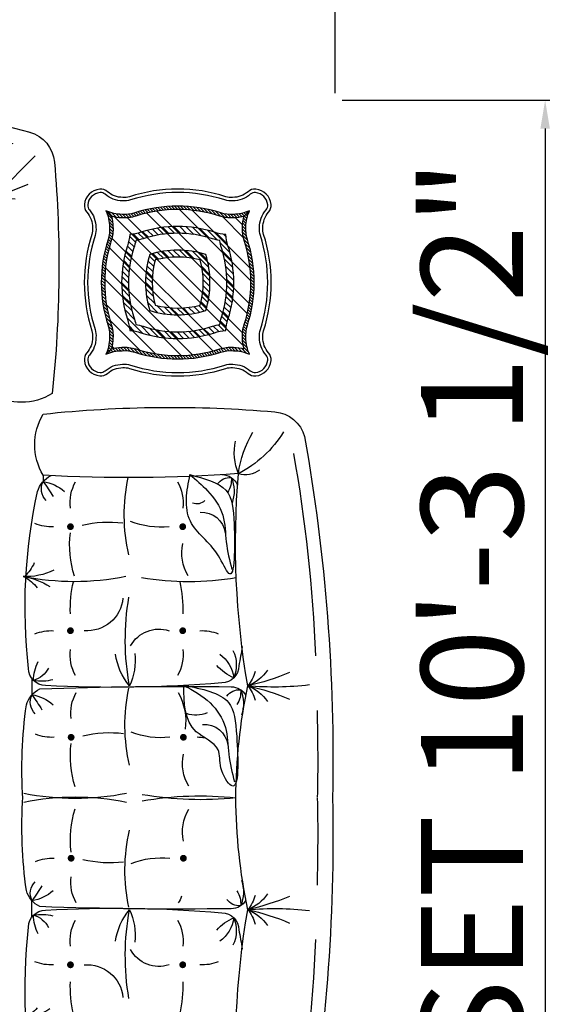
# Model space of a CAD drawing. Units: inches. Extents: x 3592 to 4861, y 1650 to 2243.
# Tile 10 of 30: x 4219 to 4265, y 1916 to 2003. Entities that reach past the tile are written whole.
import ezdxf

# ---------------------------------------------------------------- set-up
doc = ezdxf.new("R2010")
doc.units = ezdxf.units.IN
doc.layers.add('A-ANNO-DIMS', color=2, linetype='Continuous', lineweight=13)
doc.layers.add('A-FURN', color=9, linetype='Continuous', lineweight=13)
doc.layers.add('RA-AP-01$0$FURN', color=3, linetype='Continuous')
doc.layers.add('RA-AP-01$0$WOOD', color=64, linetype='Continuous')
doc.styles.get("Standard").update_dxf_attribs({"font": 'arial.ttf'})
doc.dimstyles.new('ISO-25', dxfattribs={"dimtxt": 9, "dimasz": 2.5, "dimexe": 1.25, "dimexo": 0.625, "dimtad": 1, "dimlunit": 3, "dimtxsty": 'Standard', "dimcen": 2.5, "dimadec": 0, "dimazin": 0, "dimtfac": 1, "dimtmove": 0, "dimatfit": 3, "dimfxl": 1, "dimarcsym": 0})
pattern_1 = [(225, (10.907943, -14.206733), (0.008838835, -0.008838835), [])]
pattern_2 = [(225, (10.9079426, -14.206733), (0.0044194174, -0.0044194174), [])]

# ---------------------------------------------------------------- blocks, each defined once
blk = doc.blocks.new('A$C6E322C05')
at = {"layer": 'RA-AP-01$0$FURN'}
for p, q in [((6.3919, -6.482), (6.5167, -6.3573)), ((6.3919, -6.482), (6.4334, -6.3775)), ((6.3919, -6.482), (6.3904, -6.4155)), ((5.8172, -6.4867), (5.8172, -6.5051)), ((6.3919, -6.482), (6.4393, -6.4682)), ((5.7672, -7.0775), (5.7672, -7.1067)), ((5.7672, -7.1359), (5.7672, -7.1067)), ((5.8172, -7.7267), (5.8172, -7.7084))]:
    blk.add_line(p, q, dxfattribs=at)
at = {"layer": 'RA-AP-01$0$FURN', "const_width": 0.01}
for points in [[(5.9025, -6.6381, 1), (5.8925, -6.6381, 1)], [(6.2228, -6.6381, -1), (6.2328, -6.6381, -1)], [(5.9025, -6.9444, -1), (5.8925, -6.9444, -1)], [(6.2228, -6.9444, 1), (6.2328, -6.9444, 1)], [(5.9025, -7.269, 1), (5.8925, -7.269, 1)], [(6.2228, -7.269, -1), (6.2328, -7.269, -1)], [(5.9025, -7.5753, -1), (5.8925, -7.5753, -1)], [(6.2228, -7.5753, 1), (6.2328, -7.5753, 1)]]:
    blk.add_lwpolyline(points, format="xyb", close=True, dxfattribs=at)
at = {"layer": 'RA-AP-01$0$FURN'}
for centre, radius, start, end in [((6.1922, -9.8397), 3.5528, 85.0473, 96.0589), ((5.9622, -6.3967), 0.1707, 148.1726, 211.8274), ((6.4903, -6.3998), 0.1, 15.4995, 85.0473), ((4.3367, -6.997), 2.3349, 357.3064, 15.4995), ((4.8466, -6.9097), 1.7752, 356.478, 15.9335), ((5.8573, -6.535), 0.05, 90, 180), ((6.0683, -2.0198), 4.4739, 266.7829, 274.1477), ((6.343, -6.535), 0.05, 22.5827, 90), ((8.747, -6.6855), 2.3639, 175.063, 189.8434), ((5.86, -6.527), 0.0479, 152.8071, 225.4025), ((5.7982, -6.6254), 0.1219, 48.0376, 81.0462), ((4.9043, -7.1366), 1.1102, 31.9329, 34.6665), ((6.0178, -6.5669), 0.1214, 150.1419, 187.6917), ((6.134, -6.5955), 0.1215, 123.1053, 153.7006), ((6.5659, -6.6031), 0.5101, 167.6182, 193.3122), ((6.1475, -6.4635), 0.0853, 200.7831, 253.0462), ((6.1075, -6.5669), 0.1214, 352.3083, 29.8581), ((6.3679, -6.5411), 0.0479, 86.5753, 142.6834), ((6.3027, -6.4996), 0.0683, 326.673, 5.2184), ((6.2748, -6.5339), 0.1042, 340.4828, 22.8693), ((7.0946, -6.9193), 1.3435, 163.3777, 185.4807), ((6.2698, -6.5402), 0.031, 245.776, 317.3789), ((6.2843, -6.6645), 0.0689, 6.4195, 94.4616), ((5.8396, -6.5171), 0.1213, 247.3376, 273.7315), ((6.0116, -6.9762), 0.3517, 83.4125, 103.1675), ((6.1623, -6.3952), 0.2442, 248.9017, 275.9924), ((6.1975, -6.6925), 0.3024, 173.0945, 197.5881), ((6.3545, -6.7151), 0.1295, 167.9901, 211.3796), ((5.6503, -6.6735), 0.1579, 315.4052, 333.0845), ((5.7659, -6.5936), 0.1916, 267.5853, 295.5831), ((5.9088, -6.0346), 0.7655, 258.6273, 281.4174), ((5.7331, -6.9697), 0.1864, 56.2926, 82.3818), ((5.6794, -6.9201), 0.1579, 40.3865, 58.0658), ((6.2458, -6.8794), 0.3487, 166.8392, 182.4658), ((6.2459, -5.9772), 0.8233, 260.2449, 279.7551), ((5.8795, -6.8794), 0.3487, 357.5342, 13.1608), ((5.9595, -6.8591), 0.093, 293.6025, 6.6107), ((6.8074, -6.9716), 0.7485, 170.3094, 190.3986), ((5.8396, -7.0655), 0.1213, 86.2685, 112.6624), ((5.9673, -7.035), 0.0954, 28.8034, 108.2253), ((6.158, -7.035), 0.0954, 71.7747, 151.1966), ((6.2857, -7.0655), 0.1213, 67.3376, 93.7315), ((6.0178, -7.0157), 0.1214, 172.3083, 209.8581), ((6.1075, -7.0157), 0.1214, 330.1419, 7.6917), ((6.28, -7.0949), 0.0991, 6.9226, 55.1088), ((6.2863, -7.0456), 0.0993, 337.9047, 25.6344), ((5.087, -6.7913), 1.3309, 348.8964, 351.3771), ((5.9042, -7.0857), 0.1324, 153.8888, 178.8007), ((6.2111, -6.9471), 0.2123, 205.9704, 228.742), ((5.9995, -7.0211), 0.1117, 309.9426, 354.6906), ((5.8073, -7.0476), 0.05, 180, 270), ((5.7515, -7.0133), 0.0726, 286.3559, 332.6775), ((6.4323, -6.9553), 0.1386, 221.2289, 247.0868), ((6.343, -7.0476), 0.05, 270, 360), ((6.3046, -7.0248), 0.1411, 324.485, 351.7973), ((6.3746, -6.8181), 0.292, 278.8152, 302.6921), ((6.2856, -6.8652), 0.2761, 298.9826, 313.6694), ((5.7956, -6.9527), 0.1324, 259.6959, 284.6078), ((6.0752, -3.1637), 3.943, 266.1043, 273.8957), ((6.3194, -7.1067), 0.1, 350.1566, 9.8434), ((5.8073, -7.1658), 0.05, 90, 180), ((5.7956, -7.2607), 0.1324, 75.3922, 100.3041), ((5.9042, -7.1277), 0.1324, 181.1993, 206.1112), ((5.7515, -7.2001), 0.0726, 27.3225, 73.6441), ((6.0752, -11.0497), 3.943, 86.1043, 93.8957), ((6.2139, -7.2252), 0.1855, 140.3168, 172.0523), ((6.8074, -7.2418), 0.7485, 169.6011, 189.6906), ((5.9113, -7.1825), 0.1769, 353.6796, 25.3608), ((6.4323, -7.2581), 0.1386, 112.9132, 138.7711), ((6.28, -7.1185), 0.0991, 304.8912, 353.0774), ((6.343, -7.1658), 0.05, 0, 90), ((6.2863, -7.1678), 0.0993, 334.3656, 22.0953), ((8.747, -7.5279), 2.3639, 170.1566, 184.937), ((6.4964, -7.9619), 0.8587, 83.0376, 95.1445), ((6.3757, -7.2207), 0.122, 33.7136, 69.041), ((6.3383, -7.1753), 0.1062, 14.3648, 40.2303), ((6.2695, -7.7891), 0.6986, 67.0091, 77.612), ((4.3367, -7.2164), 2.3349, 344.5005, 2.6936), ((6.0178, -7.1977), 0.1214, 150.1419, 187.6917), ((6.1075, -7.1977), 0.1214, 352.3083, 29.8581), ((7.291, -7.294), 1.5391, 175.2234, 194.4661), ((5.087, -7.4221), 1.3309, 8.6229, 11.1036), ((4.8466, -7.3037), 1.7752, 344.0665, 3.522), ((6.158, -7.1784), 0.0954, 208.8034, 288.2253), ((5.8396, -7.1479), 0.1213, 247.3376, 273.7315), ((5.9463, -7.3746), 0.106, 5.1859, 94.8073), ((6.2857, -7.1479), 0.1213, 266.2685, 292.6624), ((6.2458, -7.334), 0.3487, 177.5342, 193.1608), ((5.8795, -7.334), 0.3487, 346.8392, 2.4658), ((5.7331, -7.2437), 0.1864, 277.6182, 303.7074), ((5.9088, -8.1788), 0.7655, 78.5826, 101.3727), ((5.6794, -7.2933), 0.1579, 301.9342, 319.6135), ((6.2459, -8.2362), 0.8233, 80.2449, 99.7551), ((5.7659, -7.6198), 0.1916, 64.4169, 92.4147), ((5.6503, -7.5399), 0.1579, 26.9155, 44.5948), ((6.1975, -7.5209), 0.3024, 162.4119, 186.9055), ((6.3545, -7.4983), 0.1295, 148.6204, 192.0099), ((6.5659, -7.6103), 0.5101, 166.6878, 192.3818), ((6.2843, -7.5489), 0.0689, 265.5384, 353.5805), ((5.8396, -7.6963), 0.1213, 86.2685, 112.6624), ((6.0116, -7.2373), 0.3517, 256.8325, 276.5875), ((6.1623, -7.8182), 0.2442, 84.0076, 111.0983), ((5.86, -7.6864), 0.0479, 134.5975, 207.1929), ((6.0178, -7.6465), 0.1214, 172.3083, 209.8581), ((6.1075, -7.6465), 0.1214, 330.1419, 7.6917), ((6.2698, -7.6732), 0.031, 42.6211, 114.224), ((6.2748, -7.6795), 0.1042, 337.1307, 19.5172), ((5.8732, -7.6577), 0.0754, 196.0166, 244.1254), ((5.7982, -7.588), 0.1219, 278.9538, 311.9624), ((4.9043, -7.0769), 1.1102, 325.3335, 328.0671), ((6.3027, -7.7138), 0.0683, 354.7816, 33.327), ((6.3679, -7.6723), 0.0479, 217.3166, 273.4247), ((6.343, -7.6785), 0.05, 270, 337.4173), ((5.9667, -7.8167), 0.1745, 148.9518, 211.0482), ((6.0683, -12.1936), 4.4739, 85.8523, 93.2171), ((6.5496, -7.7946), 0.1699, 158.1488, 191.1222), ((6.4123, -7.7988), 0.0705, 53.5874, 106.8661), ((6.7131, -7.688), 0.3242, 187.6974, 210.7014), ((6.2371, -8.0321), 0.3382, 31.7436, 62.7697), ((6.4903, -7.8137), 0.1, 274.9527, 344.5005), ((6.1922, -4.3737), 3.5528, 263.9411, 274.9527)]:
    blk.add_arc(centre, radius, start, end, dxfattribs=at)
for points, knots in [([(6.2491, -6.4849), (6.2399, -6.5334), (6.2266, -6.6036), (6.2907, -6.674), (6.3321, -6.7134), (6.3818, -6.8312), (6.3817, -6.6297), (6.3708, -6.5166), (6.2912, -6.4959), (6.2491, -6.4849)], [0, 0, 0, 0, 0.1367587, 0.1981302, 0.267773, 0.3281195, 0.4737578, 0.5765194, 0.6920332, 0.6920332, 0.6920332, 0.6920332]), ([(6.2491, -6.4849), (6.2669, -6.4999), (6.3062, -6.533), (6.3538, -6.6001), (6.3525, -6.6851), (6.3659, -6.7377), (6.3727, -6.7646)], [0, 0, 0, 0, 0.0700185, 0.155078, 0.2344492, 0.3178049, 0.3178049, 0.3178049, 0.3178049]), ([(6.2491, -7.7285), (6.2399, -7.6801), (6.2266, -7.6099), (6.2907, -7.5394), (6.3321, -7.5001), (6.3818, -7.3822), (6.3817, -7.5838), (6.3708, -7.6968), (6.2912, -7.7175), (6.2491, -7.7285)], [0, 0, 0, 0, 0.1367587, 0.1981302, 0.267773, 0.3281195, 0.4737578, 0.5765194, 0.6920332, 0.6920332, 0.6920332, 0.6920332]), ([(6.2491, -7.7285), (6.2669, -7.7136), (6.3062, -7.6804), (6.3538, -7.6133), (6.3525, -7.5283), (6.3659, -7.4757), (6.3727, -7.4488)], [0, 0, 0, 0, 0.0700185, 0.155078, 0.2344492, 0.3178049, 0.3178049, 0.3178049, 0.3178049])]:
    blk.add_open_spline(points, degree=3, knots=knots, dxfattribs=at)
blk = doc.blocks.new('A$C7EE91E48')
at = {"layer": 'RA-AP-01$0$FURN'}
for p, q in [((8.4752, -8.8836), (8.5044, -8.8836)), ((8.5044, -8.8836), (8.5227, -8.8836)), ((9.1476, -8.8836), (9.1292, -8.8836)), ((9.1768, -8.8836), (9.1476, -8.8836)), ((7.8765, -8.9166), (7.8948, -8.9166)), ((9.7755, -8.9166), (9.7571, -8.9166))]:
    blk.add_line(p, q, dxfattribs=at)
at = {"layer": 'RA-AP-01$0$FURN', "const_width": 0.01}
for points in [[(8.0279, -9.0019, -1), (8.0279, -8.9919, -1)], [(8.3342, -9.0019, 1), (8.3342, -8.9919, 1)], [(8.6479, -9.0039, -1), (8.6479, -8.9939, -1)], [(9.004, -9.0039, 1), (9.004, -8.9939, 1)], [(9.3177, -9.0019, -1), (9.3177, -8.9919, -1)], [(9.624, -9.0019, 1), (9.624, -8.9919, 1)], [(8.0279, -9.3223, 1), (8.0279, -9.3323, 1)], [(8.3342, -9.3223, -1), (8.3342, -9.3323, -1)], [(8.6479, -9.3243, 1), (8.6479, -9.3343, 1)], [(9.004, -9.3243, -1), (9.004, -9.3343, -1)], [(9.3177, -9.3223, 1), (9.3177, -9.3323, 1)], [(9.624, -9.3223, -1), (9.624, -9.3323, -1)]]:
    blk.add_lwpolyline(points, format="xyb", close=True, dxfattribs=at)
at = {"layer": 'RA-AP-01$0$FURN'}
for centre, radius, start, end in [((8.2641, -10.4424), 1.5791, 83.4116, 102.408), ((8.0633, -8.7497), 0.1579, 296.9155, 314.5948), ((7.9834, -8.8653), 0.1916, 334.4169, 2.4147), ((7.4244, -9.0082), 0.7655, 348.5826, 11.3727), ((8.3595, -8.8326), 0.1864, 187.6182, 213.7074), ((8.3098, -8.7788), 0.1579, 211.9342, 229.6135), ((8.5734, -8.9396), 0.0754, 106.0166, 154.1254), ((8.744, -10.2748), 1.4207, 86.5948, 97.7424), ((8.0629, -9.0102), 0.7655, 348.5826, 11.3727), ((8.9079, -10.2748), 1.4207, 82.2576, 93.4052), ((9.589, -9.0102), 0.7655, 168.6273, 191.4174), ((9.0785, -8.9396), 0.0754, 25.8746, 73.9834), ((9.3879, -10.4424), 1.5791, 77.592, 96.5884), ((9.3421, -8.7788), 0.1579, 310.3865, 328.0658), ((9.2924, -8.8326), 0.1864, 326.2926, 352.3818), ((10.2276, -9.0082), 0.7655, 168.6273, 191.4174), ((9.6686, -8.8653), 0.1916, 177.5853, 205.5831), ((9.5886, -8.7497), 0.1579, 225.4052, 243.0845), ((7.7865, -9.0661), 0.1745, 58.9518, 121.0482), ((7.9069, -8.939), 0.1213, 356.2685, 22.6624), ((8.4553, -8.939), 0.1213, 157.3376, 183.7315), ((8.4834, -9.0206), 0.1324, 91.1993, 116.1112), ((8.411, -8.8679), 0.0726, 297.3225, 343.6441), ((8.4452, -8.9237), 0.05, 0, 90), ((8.3504, -8.912), 0.1324, 345.3922, 10.3041), ((8.5446, -8.9264), 0.0479, 44.5975, 117.1929), ((8.6431, -8.8646), 0.1219, 188.9538, 221.9624), ((9.1542, -7.9707), 1.1102, 235.3335, 238.0671), ((8.5269, -8.941), 0.1213, 356.2685, 22.6624), ((9.1251, -8.941), 0.1213, 157.3376, 183.7315), ((9.1073, -8.9264), 0.0479, 62.8071, 135.4025), ((8.4977, -7.9707), 1.1102, 301.9329, 304.6665), ((9.0089, -8.8646), 0.1219, 318.0376, 351.0462), ((9.2067, -8.9237), 0.05, 90, 180), ((9.3016, -8.912), 0.1324, 169.6959, 194.6078), ((9.1686, -9.0206), 0.1324, 63.8888, 88.8007), ((9.241, -8.8679), 0.0726, 196.3559, 242.6775), ((9.1967, -8.939), 0.1213, 356.2685, 22.6624), ((9.7451, -8.939), 0.1213, 157.3376, 183.7315), ((9.8655, -9.0661), 0.1745, 58.9518, 121.0482), ((11.2294, -9.2916), 3.5528, 173.9411, 184.9527), ((3.4096, -9.1677), 4.4739, 355.8523, 3.2171), ((7.9455, -8.9726), 0.0754, 106.0166, 154.1254), ((8.0152, -8.8976), 0.1219, 188.9538, 221.9624), ((7.9168, -8.9594), 0.0479, 44.5975, 117.1929), ((8.5263, -8.0037), 1.1102, 235.3335, 238.0671), ((4.8029, -9.1271), 3.698, 355.1082, 3.1536), ((19.2274, -9.306), 10.7293, 177.86728, 180.87576), ((-1.5755, -9.306), 10.7293, 359.12424, 2.13272), ((12.8491, -9.1271), 3.698, 176.8464, 184.8918), ((9.7352, -8.9594), 0.0479, 62.8071, 135.4025), ((9.1256, -8.0037), 1.1102, 301.9329, 304.6665), ((9.7064, -8.9726), 0.0754, 25.8746, 73.9834), ((9.6367, -8.8976), 0.1219, 318.0376, 351.0462), ((14.2423, -9.1677), 4.4739, 176.7829, 184.1477), ((6.4225, -9.2916), 3.5528, 355.0473, 6.0589), ((7.9567, -9.1172), 0.1214, 82.3083, 119.8581), ((8.0823, -9.2969), 0.3024, 72.4119, 96.9055), ((8.2692, -9.3452), 0.3487, 87.5342, 103.1608), ((8.4055, -9.1172), 0.1214, 60.1419, 97.6917), ((8.5767, -9.1192), 0.1214, 82.3083, 119.8581), ((8.7023, -9.299), 0.3024, 72.4119, 96.9055), ((8.9496, -9.299), 0.3024, 83.0945, 107.5881), ((9.0753, -9.1192), 0.1214, 60.1419, 97.6917), ((9.2465, -9.1172), 0.1214, 82.3083, 119.8581), ((9.3827, -9.3452), 0.3487, 76.8392, 92.4658), ((9.5696, -9.2969), 0.3024, 83.0945, 107.5881), ((9.6953, -9.1172), 0.1214, 60.1419, 97.6917), ((8.3659, -9.111), 0.3517, 166.8325, 186.5875), ((8.2285, -9.0458), 0.106, 275.1859, 4.8073), ((8.9859, -9.113), 0.3517, 166.8325, 186.5875), ((8.666, -9.113), 0.3517, 353.4125, 13.1675), ((9.4234, -9.0458), 0.106, 175.1927, 264.8141), ((9.286, -9.111), 0.3517, 353.4125, 13.1675), ((8.378, -9.3133), 0.1855, 50.3168, 82.0523), ((9.2739, -9.3133), 0.1855, 97.9477, 129.6832), ((7.9929, -9.6653), 0.5101, 76.6878, 102.3818), ((8.3614, -9.9068), 0.7485, 79.6011, 99.6906), ((8.6129, -9.6673), 0.5101, 76.6878, 102.3818), ((9.0391, -9.6673), 0.5101, 77.6182, 103.3122), ((9.2906, -9.9068), 0.7485, 80.3094, 100.3989), ((9.6591, -9.6653), 0.5101, 77.6182, 103.3122), ((7.785, -9.2618), 0.2442, 354.0076, 21.0983), ((8.4248, -9.2574), 0.0954, 118.8034, 198.2253), ((8.4207, -9.0107), 0.1769, 263.6796, 295.3608), ((8.405, -9.2638), 0.2442, 354.0076, 21.0983), ((9.2469, -9.2638), 0.2442, 158.9017, 185.9924), ((9.2312, -9.0107), 0.1769, 244.6392, 276.3204), ((9.2271, -9.2574), 0.0954, 341.7747, 61.1966), ((9.8669, -9.2618), 0.2442, 158.9017, 185.9924), ((7.367, -9.3453), 0.8233, 350.2449, 9.7551), ((7.8327, -9.3782), 0.9989, 353.9343, 9.823), ((9.8193, -9.3782), 0.9989, 170.177, 186.0657), ((10.285, -9.3453), 0.8233, 170.2449, 189.7551), ((7.9567, -9.2069), 0.1214, 240.1419, 277.6917), ((8.1048, -9.4539), 0.1295, 58.6204, 102.0099), ((8.2692, -8.9789), 0.3487, 256.8392, 272.4658), ((8.4055, -9.2069), 0.1214, 262.3083, 299.8581), ((8.6002, -9.1634), 0.1726, 240.9024, 278.0073), ((8.7248, -9.456), 0.1295, 58.6204, 102.0099), ((8.9271, -9.456), 0.1295, 77.9901, 121.3796), ((9.0753, -9.209), 0.1214, 289.6086, 299.8581), ((9.2465, -9.2069), 0.1214, 240.1419, 277.6917), ((9.3827, -8.9789), 0.3487, 267.5342, 283.1608), ((9.5471, -9.4539), 0.1295, 77.9901, 121.3796), ((9.6953, -9.2069), 0.1214, 262.3083, 299.8581), ((7.93, -9.3692), 0.031, 312.6211, 24.224), ((8.5004, -9.3657), 0.0825, 335.8161, 19.2747), ((9.722, -9.3692), 0.031, 155.776, 227.3789), ((8.0543, -9.3837), 0.0689, 175.5384, 263.5805), ((8.4553, -9.3851), 0.1213, 176.2685, 202.6624), ((8.6789, -9.3912), 0.0689, 175.5384, 263.5805), ((8.405, -9.3948), 0.2442, 0.7304, 5.9924), ((9.1967, -9.3851), 0.1213, 337.3376, 3.7315), ((9.5977, -9.3837), 0.0689, 276.4195, 4.4616), ((7.9247, -9.4424), 0.05, 180, 247.4173), ((7.9309, -9.4673), 0.0479, 127.3166, 183.4247), ((8.4847, -9.3794), 0.0991, 214.8912, 263.0774), ((8.3451, -9.5317), 0.1386, 22.9132, 48.7711), ((8.4374, -9.4424), 0.05, 270, 0), ((9.2146, -9.4424), 0.05, 180, 270), ((9.3068, -9.5317), 0.1386, 131.2289, 157.0868), ((9.1673, -9.3794), 0.0991, 276.9226, 325.1088), ((9.7272, -9.4424), 0.05, 292.5827, 360), ((9.721, -9.4673), 0.0479, 356.5753, 52.6834), ((7.8894, -9.4022), 0.0683, 264.7816, 303.327), ((7.9236, -9.3742), 0.1042, 247.1307, 289.5172), ((8.4354, -9.3857), 0.0993, 244.3656, 292.0953), ((8.5494, -9.4699), 0.05, 180, 239.8522), ((8.5556, -9.4948), 0.0479, 127.3166, 183.4247), ((9.0963, -9.4948), 0.0479, 356.5753, 52.6834), ((9.1025, -9.4699), 0.05, 300.1478, 360), ((9.2166, -9.3857), 0.0993, 247.9047, 295.6344), ((9.7283, -9.3742), 0.1042, 250.4828, 292.8693), ((9.7626, -9.4022), 0.0683, 236.673, 275.2184), ((7.5711, -9.3365), 0.3382, 301.7436, 332.7697), ((7.9152, -9.8125), 0.3242, 97.6974, 120.7014), ((7.8086, -9.649), 0.1699, 68.1488, 101.1222), ((7.8044, -9.5117), 0.0705, 323.5874, 16.8661), ((8.0772, -11.9348), 2.4522, 80.1542, 94.8039), ((8.1811, -8.1864), 1.3309, 278.6229, 281.1036), ((8.8331, -11.1187), 1.6349, 90.2483, 101.88), ((8.514, -9.4297), 0.0683, 264.7816, 303.327), ((8.5483, -9.4017), 0.1042, 247.1307, 289.5172), ((8.8189, -11.1187), 1.6349, 78.12, 89.7517), ((9.1036, -9.4017), 0.1042, 250.4828, 292.8693), ((9.1379, -9.4297), 0.0683, 236.673, 275.2184), ((9.5748, -11.9348), 2.4522, 85.1961, 99.8458), ((9.4709, -8.1864), 1.3309, 258.8964, 261.3771), ((9.8476, -9.5117), 0.0705, 163.1339, 216.4126), ((9.8434, -9.649), 0.1699, 78.8778, 111.8512), ((9.7367, -9.8125), 0.3242, 59.2986, 82.3026), ((10.0809, -9.3365), 0.3382, 207.2303, 238.2564), ((8.3825, -9.4751), 0.122, 303.7136, 339.041), ((8.4279, -9.4377), 0.1062, 284.3648, 310.2303), ((7.8141, -9.3689), 0.6986, 337.0091, 347.612), ((7.6413, -9.5958), 0.8587, 353.0376, 5.1445), ((8.6105, -9.4751), 0.122, 200.959, 236.2864), ((8.5651, -9.4377), 0.1062, 229.7697, 255.6352), ((9.1788, -9.3689), 0.6986, 192.388, 202.9909), ((9.0415, -9.4751), 0.122, 303.7136, 339.041), ((9.0869, -9.4377), 0.1062, 284.3648, 310.2303), ((8.4731, -9.3689), 0.6986, 337.0091, 347.612), ((10.0107, -9.5958), 0.8587, 174.8555, 186.9624), ((9.2694, -9.4751), 0.122, 200.959, 236.2864), ((9.224, -9.4377), 0.1062, 229.7697, 255.6352), ((9.8378, -9.3689), 0.6986, 192.388, 202.9909), ((7.7895, -9.5897), 0.1, 184.9527, 254.5005), ((9.8624, -9.5897), 0.1, 285.4995, 355.0473), ((8.5724, -5.4361), 4.2848, 259.7801, 267.8084), ((9.0796, -5.4361), 4.2848, 272.1916, 280.2199), ((8.7159, -4.2841), 5.4854, 259.9939, 271.1496), ((8.936, -4.2841), 5.4854, 268.8504, 280.0061), ((8.7159, -4.2841), 5.4404, 268.4485, 271.1496), ((8.936, -4.2841), 5.4404, 268.8504, 271.5515)]:
    blk.add_arc(centre, radius, start, end, dxfattribs=at)
for points, knots in [([(7.8747, -9.3485), (7.9231, -9.3393), (7.9933, -9.326), (8.0638, -9.3901), (8.1031, -9.4315), (8.221, -9.4812), (8.0194, -9.4811), (7.9064, -9.4702), (7.8857, -9.3906), (7.8747, -9.3485)], [0, 0, 0, 0, 0.1367587, 0.1981302, 0.267773, 0.3281195, 0.4737578, 0.5765194, 0.6920332, 0.6920332, 0.6920332, 0.6920332]), ([(8.4947, -9.3305), (8.5098, -9.3579), (8.5387, -9.4102), (8.6151, -9.4603), (8.6994, -9.4595), (8.7521, -9.4728), (8.7791, -9.4797)], [0, 0, 0, 0, 0.0929945, 0.178054, 0.2574251, 0.3407808, 0.3407808, 0.3407808, 0.3407808]), ([(8.4947, -9.3305), (8.547, -9.3311), (8.63, -9.3319), (8.67, -9.4425), (8.7389, -9.4316), (8.8424, -9.4963), (8.6448, -9.4874), (8.5233, -9.4759), (8.5051, -9.3838), (8.4947, -9.3305)], [0, 0, 0, 0, 0.1415752, 0.2249019, 0.2789443, 0.3392908, 0.4849291, 0.5876907, 0.7285367, 0.7285367, 0.7285367, 0.7285367]), ([(9.7773, -9.3485), (9.7288, -9.3393), (9.6586, -9.326), (9.5882, -9.3901), (9.5488, -9.4315), (9.4309, -9.4812), (9.6325, -9.4811), (9.7455, -9.4702), (9.7663, -9.3906), (9.7773, -9.3485)], [0, 0, 0, 0, 0.1367587, 0.1981302, 0.267773, 0.3281195, 0.4737578, 0.5765194, 0.6920332, 0.6920332, 0.6920332, 0.6920332]), ([(7.8747, -9.3485), (7.8896, -9.3663), (7.9228, -9.4056), (7.9899, -9.4532), (8.0749, -9.4519), (8.1275, -9.4653), (8.1544, -9.4722)], [0, 0, 0, 0, 0.0700185, 0.155078, 0.2344492, 0.3178049, 0.3178049, 0.3178049, 0.3178049]), ([(9.7773, -9.3485), (9.7623, -9.3663), (9.7292, -9.4056), (9.662, -9.4532), (9.577, -9.4519), (9.5245, -9.4653), (9.4975, -9.4722)], [0, 0, 0, 0, 0.0700185, 0.155078, 0.2344492, 0.3178049, 0.3178049, 0.3178049, 0.3178049])]:
    blk.add_open_spline(points, degree=3, knots=knots, dxfattribs=at)
blk = doc.blocks.new('A$C3E710961')
at = {"layer": 'RA-AP-01$0$WOOD'}
h = blk.add_hatch(dxfattribs=at)
h.set_pattern_fill('ANSI31', color=256, scale=0.05, angle=180, style=0)
h.set_pattern_definition(pattern_2)
h.paths.add_polyline_path([(5.8026, -7.4494, 0.094014), (5.8075, -7.4087, 0.060627), (5.8033, -7.3781, 0.060627), (5.8339, -7.3823, 0.094014), (5.8746, -7.3774, -0.130533), (6.0799, -7.3664), (6.0868, -7.3576, 0.133623), (5.8716, -7.3679, -0.094597), (5.8343, -7.3723, -0.104317), (5.7868, -7.3616, -0.104317), (5.7975, -7.4091, -0.094597), (5.7931, -7.4464, 0.158024), (5.7931, -7.6995, -0.094597), (5.7975, -7.7367, -0.104317), (5.7868, -7.7842, -0.104317), (5.8343, -7.7736, -0.094597), (5.8716, -7.778, 0.158024), (6.1247, -7.778, -0.094597), (6.1619, -7.7736, -0.104317), (6.2094, -7.7842, -0.104317), (6.1987, -7.7367, -0.094597), (6.2031, -7.6995, 0.158024), (6.2031, -7.4464, -0.094597), (6.1987, -7.4091, -0.104317), (6.2094, -7.3616, -0.104317), (6.1619, -7.3723, -0.094597), (6.1247, -7.3679, 0.023897), (6.0868, -7.3576), (6.0799, -7.3664, -0.026981), (6.1216, -7.3774, 0.094014), (6.1623, -7.3823, 0.060627), (6.193, -7.3781, 0.060627), (6.1888, -7.4087, 0.094014), (6.1936, -7.4494, -0.158071), (6.1936, -7.6964, 0.094014), (6.1888, -7.7372, 0.060627), (6.193, -7.7678, 0.060627), (6.1623, -7.7636, 0.094014), (6.1216, -7.7684, -0.158071), (5.8746, -7.7684, 0.094014), (5.8339, -7.7636, 0.060627), (5.8033, -7.7678, 0.060627), (5.8075, -7.7372, 0.094014), (5.8026, -7.6964, -0.158071)])
h = blk.add_hatch(dxfattribs=at)
h.set_pattern_fill('ANSI31', color=256, scale=0.05, angle=180, style=0)
h.set_pattern_definition(pattern_2)
h.paths.add_polyline_path([(5.8026, -7.4494, 0.094014), (5.8075, -7.4087, 0.060627), (5.8033, -7.3781, 0.060627), (5.8339, -7.3823, 0.094014), (5.8746, -7.3774, -0.130533), (6.0799, -7.3664), (6.0868, -7.3576, 0.133623), (5.8716, -7.3679, -0.094597), (5.8343, -7.3723, -0.104317), (5.7868, -7.3616, -0.104317), (5.7975, -7.4091, -0.094597), (5.7931, -7.4464, 0.158024), (5.7931, -7.6995, -0.094597), (5.7975, -7.7367, -0.104317), (5.7868, -7.7842, -0.104317), (5.8343, -7.7736, -0.094597), (5.8716, -7.778, 0.158024), (6.1247, -7.778, -0.094597), (6.1619, -7.7736, -0.104317), (6.2094, -7.7842, -0.104317), (6.1987, -7.7367, -0.094597), (6.2031, -7.6995, 0.158024), (6.2031, -7.4464, -0.094597), (6.1987, -7.4091, -0.104317), (6.2094, -7.3616, -0.104317), (6.1619, -7.3723, -0.094597), (6.1247, -7.3679, 0.023897), (6.0868, -7.3576), (6.0799, -7.3664, -0.026981), (6.1216, -7.3774, 0.094014), (6.1623, -7.3823, 0.060627), (6.193, -7.3781, 0.060627), (6.1888, -7.4087, 0.094014), (6.1936, -7.4494, -0.158071), (6.1936, -7.6964, 0.094014), (6.1888, -7.7372, 0.060627), (6.193, -7.7678, 0.060627), (6.1623, -7.7636, 0.094014), (6.1216, -7.7684, -0.158071), (5.8746, -7.7684, 0.094014), (5.8339, -7.7636, 0.060627), (5.8033, -7.7678, 0.060627), (5.8075, -7.7372, 0.094014), (5.8026, -7.6964, -0.158071)])
h = blk.add_hatch(dxfattribs=at)
h.set_pattern_fill('ANSI32,_I', color=256, scale=0.2, angle=180, style=2)
h.set_pattern_definition([(225, (-0.32707, -3.57881), (0.053033, -0.053033), []), (225, (-0.36242, -3.57881), (0.053033, -0.053033), [])])
h.paths.add_polyline_path([(5.8693, -7.675, -0.030626), (5.8746, -7.6964, -0.030626), (5.896, -7.7018, 0.158398), (6.1002, -7.7018, -0.030626), (6.1216, -7.6964, -0.030626), (6.127, -7.675, 0.158398), (6.127, -7.4708, -0.030626), (6.1216, -7.4495, -0.030626), (6.1002, -7.4441, 0.158398), (5.896, -7.4441, -0.030626), (5.8746, -7.4495, -0.030626), (5.8693, -7.4708, 0.158398)], flags=16)
h.paths.add_polyline_path([(5.8026, -7.6964, -0.094014), (5.8075, -7.7372, -0.060627), (5.8033, -7.7678, -0.060627), (5.8339, -7.7636, -0.094014), (5.8746, -7.7684, 0.158071), (6.1216, -7.7684, -0.094014), (6.1623, -7.7636, -0.060627), (6.193, -7.7678, -0.060627), (6.1888, -7.7372, -0.094014), (6.1936, -7.6964, 0.158071), (6.1936, -7.4494, -0.094014), (6.1888, -7.4087, -0.060627), (6.193, -7.3781, -0.060627), (6.1623, -7.3823, -0.094014), (6.1216, -7.3774, 0.158071), (5.8746, -7.3774, -0.094014), (5.8339, -7.3823, -0.060627), (5.8033, -7.3781, -0.060627), (5.8075, -7.4087, -0.094014), (5.8026, -7.4494, 0.158071)])
h.paths.add_polyline_path([(5.8693, -7.4708, 0.030626), (5.8746, -7.4495, 0.030626), (5.896, -7.4441, -0.158398), (6.1002, -7.4441, 0.030626), (6.1216, -7.4495, 0.030626), (6.127, -7.4708, -0.158398), (6.127, -7.675, 0.030626), (6.1216, -7.6964, 0.030626), (6.1002, -7.7018, -0.158398), (5.896, -7.7018, 0.030626), (5.8746, -7.6964, 0.030626), (5.8693, -7.675, -0.158398)], flags=0)
h = blk.add_hatch(dxfattribs=at)
h.set_pattern_fill('ANSI31', color=256, scale=0.1, angle=180, style=0)
h.set_pattern_definition(pattern_1)
h.paths.add_polyline_path([(5.8693, -7.675, -0.158398), (5.8693, -7.4708, 0.030626), (5.8746, -7.4495, 0.030626), (5.896, -7.4441, -0.102814), (6.0297, -7.4294), (6.0443, -7.411, 0.112048), (5.8899, -7.425, -0.052642), (5.857, -7.4318, -0.052642), (5.8502, -7.4647, 0.158303), (5.8502, -7.6812, -0.052642), (5.857, -7.7141, -0.052642), (5.8899, -7.7208, 0.0216), (5.919, -7.7289), (5.9329, -7.7115, -0.028915), (5.896, -7.7018, 0.030626), (5.8746, -7.6964, 0.030626)])
h.paths.add_polyline_path([(5.9329, -7.7115), (5.919, -7.7289, 0.136237), (6.1063, -7.7208, -0.052642), (6.1392, -7.7141, -0.052642), (6.146, -7.6812, 0.158303), (6.146, -7.4647, -0.052642), (6.1392, -7.4318, -0.052642), (6.1063, -7.425, 0.045448), (6.0443, -7.411), (6.0297, -7.4294, -0.054693), (6.1002, -7.4441, 0.030626), (6.1216, -7.4495, 0.030626), (6.127, -7.4708, -0.158398), (6.127, -7.675, 0.030626), (6.1216, -7.6964, 0.030626), (6.1002, -7.7018, -0.128893)])
h.paths.add_polyline_path([(6.0645, -7.6394, -0.078369), (5.9838, -7.6476), (5.9688, -7.6664, 0.101268), (6.0807, -7.6555, 0.125365), (6.0875, -7.5173), (6.0708, -7.5383, -0.098159)], flags=17)
h.paths.add_polyline_path([(6.0645, -7.5065, -0.031109), (6.0708, -7.5383), (6.0875, -7.5173, 0.024773), (6.0807, -7.4904, 0.081275), (5.991, -7.478), (5.9743, -7.499, -0.087626)], flags=17)
h.paths.add_polyline_path([(5.9155, -7.4904, 0.150605), (5.9155, -7.6555, 0.048597), (5.9688, -7.6664), (5.9838, -7.6476, -0.05078), (5.9317, -7.6394, -0.129665), (5.9317, -7.5065, -0.041567), (5.9743, -7.499), (5.991, -7.478, 0.068492)], flags=17)
h = blk.add_hatch(dxfattribs=at)
h.set_pattern_fill('ANSI31', color=256, scale=0.1, angle=180, style=0)
h.set_pattern_definition(pattern_1)
h.paths.add_polyline_path([(5.8693, -7.675, -0.158398), (5.8693, -7.4708, 0.030626), (5.8746, -7.4495, 0.030626), (5.896, -7.4441, -0.102814), (6.0297, -7.4294), (6.0443, -7.411, 0.112048), (5.8899, -7.425, -0.052642), (5.857, -7.4318, -0.052642), (5.8502, -7.4647, 0.158303), (5.8502, -7.6812, -0.052642), (5.857, -7.7141, -0.052642), (5.8899, -7.7208, 0.0216), (5.919, -7.7289), (5.9329, -7.7115, -0.028915), (5.896, -7.7018, 0.030626), (5.8746, -7.6964, 0.030626)])
h.paths.add_polyline_path([(5.9329, -7.7115), (5.919, -7.7289, 0.136237), (6.1063, -7.7208, -0.052642), (6.1392, -7.7141, -0.052642), (6.146, -7.6812, 0.158303), (6.146, -7.4647, -0.052642), (6.1392, -7.4318, -0.052642), (6.1063, -7.425, 0.045448), (6.0443, -7.411), (6.0297, -7.4294, -0.054693), (6.1002, -7.4441, 0.030626), (6.1216, -7.4495, 0.030626), (6.127, -7.4708, -0.158398), (6.127, -7.675, 0.030626), (6.1216, -7.6964, 0.030626), (6.1002, -7.7018, -0.128893)])
h.paths.add_polyline_path([(6.0645, -7.6394, -0.078369), (5.9838, -7.6476), (5.9688, -7.6664, 0.101268), (6.0807, -7.6555, 0.125365), (6.0875, -7.5173), (6.0708, -7.5383, -0.098159)], flags=17)
h.paths.add_polyline_path([(6.0645, -7.5065, -0.031109), (6.0708, -7.5383), (6.0875, -7.5173, 0.024773), (6.0807, -7.4904, 0.081275), (5.991, -7.478), (5.9743, -7.499, -0.087626)], flags=17)
h.paths.add_polyline_path([(5.9155, -7.4904, 0.150605), (5.9155, -7.6555, 0.048597), (5.9688, -7.6664), (5.9838, -7.6476, -0.05078), (5.9317, -7.6394, -0.129665), (5.9317, -7.5065, -0.041567), (5.9743, -7.499), (5.991, -7.478, 0.068492)], flags=17)
for p, q in [((5.8033, -7.3781), (5.7868, -7.3616)), ((5.8033, -7.3781), (5.7868, -7.3616)), ((5.8033, -7.7678), (5.7868, -7.7842)), ((5.8033, -7.7678), (5.7868, -7.7842)), ((6.193, -7.7678), (6.2094, -7.7842)), ((6.193, -7.7678), (6.2094, -7.7842))]:
    blk.add_line(p, q, dxfattribs=at)
for points in [[(6.2052, -7.8404, 0.205661), (6.2277, -7.8477, 0.361434), (6.2729, -7.8025, 0.205661), (6.2656, -7.78, -0.184266), (6.2487, -7.7346, -0.100949), (6.2508, -7.7147, 0.157773), (6.2508, -7.4312, -0.100949), (6.2487, -7.4113, -0.184266), (6.2656, -7.3659, 0.205661), (6.2729, -7.3434, 0.361434), (6.2277, -7.2981, 0.205661), (6.2052, -7.3055, -0.184266), (6.1597, -7.3223, -0.100949), (6.1399, -7.3203, 0.157773), (5.8564, -7.3203, -0.100949), (5.8365, -7.3223, -0.184266), (5.791, -7.3055, 0.205661), (5.7685, -7.2981, 0.361434), (5.7233, -7.3434, 0.205661), (5.7306, -7.3659, -0.184266), (5.7475, -7.4113, -0.100949), (5.7454, -7.4312, 0.157773), (5.7454, -7.7147, -0.100949), (5.7475, -7.7346, -0.184266), (5.7306, -7.78, 0.205661), (5.7233, -7.8025, 0.361434), (5.7685, -7.8477, 0.205661), (5.791, -7.8404, -0.184266), (5.8365, -7.8236, -0.100949), (5.8564, -7.8256, 0.157773), (6.1399, -7.8256, -0.100949), (6.1597, -7.8236, -0.184266)], [(6.2118, -7.8329, 0.205661), (6.2268, -7.8378, 0.361434), (6.2629, -7.8016, 0.205661), (6.2581, -7.7866, -0.182482), (6.2387, -7.735, -0.098854), (6.2412, -7.7117, 0.157827), (6.2412, -7.4342, -0.098854), (6.2387, -7.4109, -0.182482), (6.2581, -7.3593, 0.205661), (6.2629, -7.3443, 0.361434), (6.2268, -7.3081, 0.205661), (6.2118, -7.313, -0.182482), (6.1602, -7.3323, -0.098854), (6.1368, -7.3298, 0.157827), (5.8594, -7.3298, -0.098854), (5.836, -7.3323, -0.182482), (5.7845, -7.313, 0.205661), (5.7694, -7.3081, 0.361434), (5.7333, -7.3443, 0.205661), (5.7382, -7.3593, -0.182482), (5.7575, -7.4109, -0.098854), (5.755, -7.4342, 0.157827), (5.755, -7.7117, -0.098854), (5.7575, -7.735, -0.182482), (5.7382, -7.7866, 0.205661), (5.7333, -7.8016, 0.361434), (5.7694, -7.8378, 0.205661), (5.7845, -7.8329, -0.182482), (5.836, -7.8136, -0.098854), (5.8594, -7.8161, 0.157827), (6.1368, -7.8161, -0.098854), (6.1602, -7.8136, -0.182482)], [(6.2094, -7.7842, -0.104317), (6.1987, -7.7367, -0.094597), (6.2031, -7.6995, 0.158024), (6.2031, -7.4464, -0.094597), (6.1987, -7.4091, -0.104317), (6.2094, -7.3616, -0.104317), (6.1619, -7.3723, -0.094597), (6.1247, -7.3679, 0.158024), (5.8716, -7.3679, -0.094597), (5.8343, -7.3723, -0.104317), (5.7868, -7.3616, -0.104317), (5.7975, -7.4091, -0.094597), (5.7931, -7.4464, 0.158024), (5.7931, -7.6995, -0.094597), (5.7975, -7.7367, -0.104317), (5.7868, -7.7842, -0.104317), (5.8343, -7.7736, -0.094597), (5.8716, -7.778, 0.158024), (6.1247, -7.778, -0.094597), (6.1619, -7.7736, -0.104317)], [(6.193, -7.7678, -0.060627), (6.1888, -7.7372, -0.094014), (6.1936, -7.6964, 0.158071), (6.1936, -7.4494, -0.094014), (6.1888, -7.4087, -0.060627), (6.193, -7.3781, -0.060627), (6.1623, -7.3823, -0.094014), (6.1216, -7.3774, 0.158071), (5.8746, -7.3774, -0.094014), (5.8339, -7.3823, -0.060627), (5.8033, -7.3781, -0.060627), (5.8075, -7.4087, -0.094014), (5.8026, -7.4494, 0.158071), (5.8026, -7.6964, -0.094014), (5.8075, -7.7372, -0.060627), (5.8033, -7.7678, -0.060627), (5.8339, -7.7636, -0.094014), (5.8746, -7.7684, 0.158071), (6.1216, -7.7684, -0.094014), (6.1623, -7.7636, -0.060627)], [(6.1392, -7.7141, -0.052642), (6.146, -7.6812, 0.158303), (6.146, -7.4647, -0.052642), (6.1392, -7.4318, -0.052642), (6.1063, -7.425, 0.158303), (5.8899, -7.425, -0.052642), (5.857, -7.4318, -0.052642), (5.8502, -7.4647, 0.158303), (5.8502, -7.6812, -0.052642), (5.857, -7.7141, -0.052642), (5.8899, -7.7208, 0.158303), (6.1063, -7.7208, -0.052642)], [(6.1216, -7.6964, -0.030626), (6.127, -7.675, 0.158398), (6.127, -7.4708, -0.030626), (6.1216, -7.4495, -0.030626), (6.1002, -7.4441, 0.158398), (5.896, -7.4441, -0.030626), (5.8746, -7.4495, -0.030626), (5.8693, -7.4708, 0.158398), (5.8693, -7.675, -0.030626), (5.8746, -7.6964, -0.030626), (5.896, -7.7018, 0.158398), (6.1002, -7.7018, -0.030626)], [(6.0807, -7.6555, 0.150605), (6.0807, -7.4904, 0.150605), (5.9155, -7.4904, 0.150605), (5.9155, -7.6555, 0.150605)], [(6.0645, -7.6394, 0.129665), (6.0645, -7.5065, 0.129665), (5.9317, -7.5065, 0.129665), (5.9317, -7.6394, 0.129665)]]:
    blk.add_lwpolyline(points, format="xyb", close=True, dxfattribs=at)
blk = doc.blocks.new('A$C44E37296')
at = {"layer": 'RA-AP-01$0$FURN'}
blk.add_blockref('A$C3E710961', (-7.4877, 9.348), dxfattribs=at)
at = {"layer": 'RA-AP-01$0$FURN', "xscale": -1}
blk.add_blockref('A$C6E322C05', (4.6545, 7.7124), dxfattribs=at)
at = {"layer": 'RA-AP-01$0$WOOD', "xscale": -1, "rotation": 180}
blk.add_blockref('A$C7EE91E48', (-8.7987, -7.5375), dxfattribs=at)
blk = doc.blocks.new('*D164')
at = {"layer": 'A-ANNO-DIMS', "color": 0, "lineweight": -2, "transparency": 16777216}
for p, q in [((4247.704, 1995.926), (4266.87, 1995.926)), ((4265.62, 1993.426), (4265.62, 1874.818)), ((4247.704, 1872.318), (4266.87, 1872.318))]:
    blk.add_line(p, q, dxfattribs=at)
at = {"layer": 'A-ANNO-DIMS', "color": 0, "transparency": 16777216}
for points in [[(4265.204, 1993.426), (4266.037, 1993.426), (4265.62, 1995.926)], [(4265.204, 1874.818), (4266.037, 1874.818), (4265.62, 1872.318)]]:
    blk.add_solid(points, dxfattribs=at)
at = {"layer": 'Defpoints', "color": 0, "transparency": 16777216}
for p in [(4247.079, 1995.926), (4247.079, 1872.318), (4265.62, 1872.318)]:
    blk.add_point(p, dxfattribs=at)
at = {"layer": 'A-ANNO-DIMS', "color": 0, "transparency": 16777216, "insert": (4260.336, 1934.122), "char_height": 9, "attachment_point": 5, "rotation": 90}
blk.add_mtext('SOFA SET 10\'-3 1/2"', dxfattribs=at)
blk = doc.blocks.new('*D165')
at = {"layer": 'A-ANNO-DIMS', "color": 0, "lineweight": -2, "transparency": 16777216}
for p, q in [((4173.347, 1996.551), (4173.347, 2015.717)), ((4247.079, 1996.551), (4247.079, 2015.717)), ((4175.847, 2014.467), (4244.579, 2014.467))]:
    blk.add_line(p, q, dxfattribs=at)
at = {"layer": 'A-ANNO-DIMS', "color": 0, "transparency": 16777216}
for points in [[(4175.847, 2014.884), (4175.847, 2014.051), (4173.347, 2014.467)], [(4244.579, 2014.884), (4244.579, 2014.051), (4247.079, 2014.467)]]:
    blk.add_solid(points, dxfattribs=at)
at = {"layer": 'Defpoints', "color": 0, "transparency": 16777216}
for p in [(4247.079, 2014.467), (4173.347, 1995.926), (4247.079, 1995.926)]:
    blk.add_point(p, dxfattribs=at)
at = {"layer": 'A-ANNO-DIMS', "color": 0, "transparency": 16777216, "insert": (4210.213, 2019.746), "char_height": 9, "attachment_point": 5}
blk.add_mtext('6\'-1 1/2"', dxfattribs=at)

msp = doc.modelspace()

# ---------------------------------------------------------------- block references
at = {"layer": 'A-FURN', "xscale": 29.98919001647196, "yscale": 29.98919001647196, "zscale": 29.98919001647196, "rotation": 270}
msp.add_blockref('A$C44E37296', (4179.961, 1935.164), dxfattribs=at)

# ---------------------------------------------------------------- dimensions: what is measured, and where the dimension line sits
at = {"layer": 'A-ANNO-DIMS'}
dim = msp.add_linear_dim(base=(4247.079, 2014.467), p1=(4173.347, 1995.926), p2=(4247.079, 1995.926), dimstyle='ISO-25', override={"dimdec": 1, "dimlfac": 1, "dimrnd": 0, "dimzin": 1, "dimdsep": 46, "dimlunit": 4, "dimfrac": 2}, dxfattribs=at)
dim.commit()
dim.dimension.update_dxf_attribs({"geometry": '*D165', "text_midpoint": (4210.213, 2019.746)})
dim = msp.add_linear_dim(base=(4265.62, 1872.318), p1=(4247.079, 1995.926), p2=(4247.079, 1872.318), angle=270, text='SOFA SET <>', dimstyle='ISO-25', override={"dimdec": 1, "dimlfac": 1, "dimrnd": 0, "dimzin": 1, "dimdsep": 46, "dimlunit": 4, "dimfrac": 2}, dxfattribs=at)
dim.commit()
dim.dimension.update_dxf_attribs({"geometry": '*D164', "text_midpoint": (4260.336, 1934.122)})

doc.saveas('drawing.dxf')
